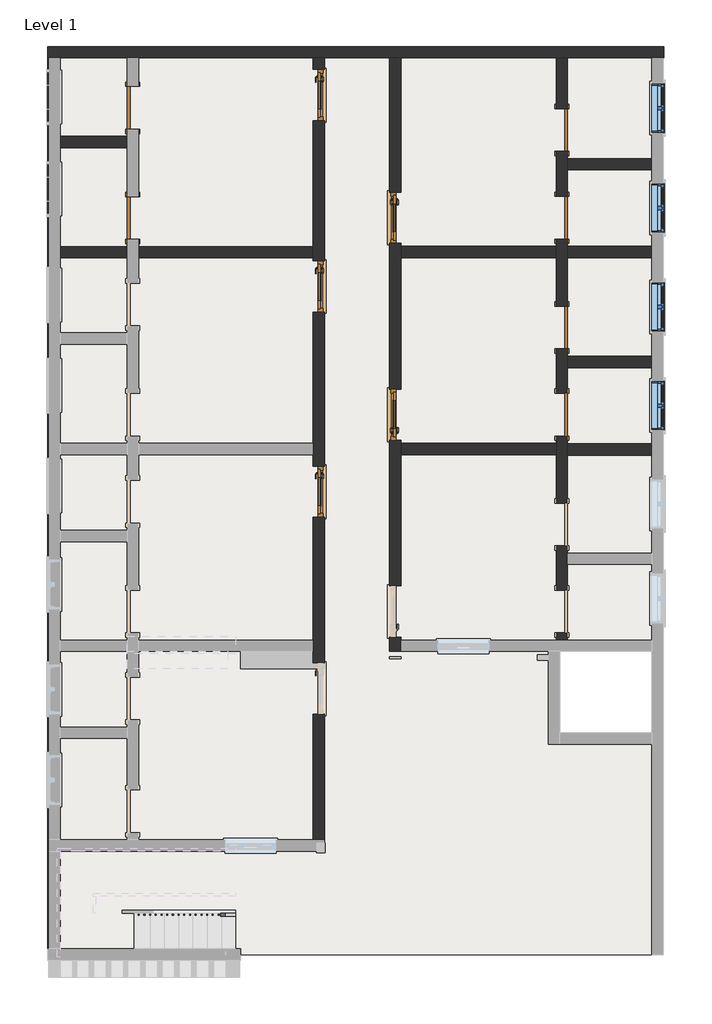
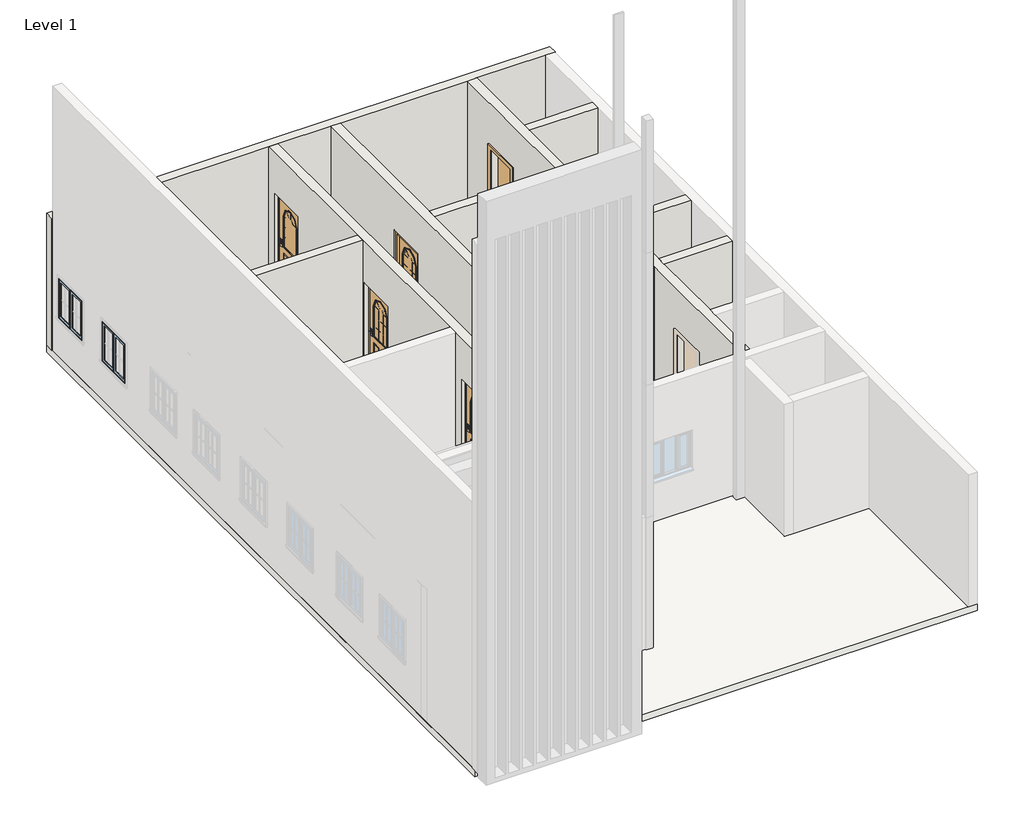
# One storey, part 2 of 4: 13 walls, 11 doors, 6 windows, 1 railing, 1 slab.
"""IFC4 building model written with IfcOpenShell, lengths in millimetres."""

from ifc_helpers import new_model, si_unit, frame, origin, origin_with_axes, place, context, project, spatial, polyline, outline, extrude, faceted_brep, transform, mapped, element, save
from components import doors_extsgl_w_glazing_bars_arched_910x2110mm_1ab485ba, doors_extsgl_w_glazing_bars_arched_910x2110mm_97dcda8a, door_53b1b562, window_c29befe5

model = new_model("IFC4")

# Units and contexts
model_context = context("Model", 3, world=origin())
ifc_project = project(units=[si_unit("LENGTHUNIT", "METRE", prefix="MILLI")], contexts=[model_context])

# Site, building, storey
site = spatial("IfcSite", under=ifc_project)
building = spatial("IfcBuilding", under=site)
storey = spatial("IfcBuildingStorey", under=building, Name="Level 1", Elevation=0.0)

# Doors
placement = place(None, origin())
doors_extsgl_w_glazing_bars_arched_910x2110mm_shape = doors_extsgl_w_glazing_bars_arched_910x2110mm_1ab485ba(model_context)
element("IfcDoor", 1, ObjectType="Doors_ExtSgl_w-Glazing_Bars_Arched : 910x2110mm", at=placement, inside=storey, context=model_context, shape_type="MappedRepresentation", body=[
    mapped(doors_extsgl_w_glazing_bars_arched_910x2110mm_shape, transform((-1635.1108866, 7135.2399728, 0.0), x_axis=(0.0, -1.0, 0.0), y_axis=(1.0, 0.0, 0.0), z_axis=(0.0, 0.0, 1.0))),
])
element("IfcDoor", 2, ObjectType="Doors_ExtSgl_w-Glazing_Bars_Arched : 910x2110mm", at=placement, inside=storey, context=model_context, shape_type="MappedRepresentation", body=[
    mapped(doors_extsgl_w_glazing_bars_arched_910x2110mm_shape, transform((-1635.1108866, 3727.1935874, 0.0), x_axis=(0.0, -1.0, 0.0), y_axis=(1.0, 0.0, 0.0), z_axis=(0.0, 0.0, 1.0))),
])
element("IfcDoor", 3, ObjectType="Doors_ExtSgl_w-Glazing_Bars_Arched : 910x2110mm", at=placement, inside=storey, context=model_context, shape_type="MappedRepresentation", body=[
    mapped(doors_extsgl_w_glazing_bars_arched_910x2110mm_shape, transform((-1635.1108866, 74.0399728, 0.0), x_axis=(0.0, -1.0, 0.0), y_axis=(1.0, 0.0, 0.0), z_axis=(0.0, 0.0, 1.0))),
])
element("IfcDoor", 4, ObjectType="Doors_ExtSgl_w-Glazing_Bars_Arched : 910x2110mm", at=placement, inside=storey, context=model_context, shape_type="MappedRepresentation", body=[
    mapped(doors_extsgl_w_glazing_bars_arched_910x2110mm_shape, transform((-276.2108866, 1445.6399728, 0.0), x_axis=(0.0, 1.0, 0.0), y_axis=(-1.0, 0.0, 0.0), z_axis=(0.0, 0.0, 1.0))),
])
doors_extsgl_w_glazing_bars_arched_910x2110mm_2_shape = doors_extsgl_w_glazing_bars_arched_910x2110mm_97dcda8a(model_context)
element("IfcDoor", 5, ObjectType="Doors_ExtSgl_w-Glazing_Bars_Arched : 910x2110mm", at=placement, inside=storey, context=model_context, shape_type="MappedRepresentation", body=[
    mapped(doors_extsgl_w_glazing_bars_arched_910x2110mm_2_shape, transform((-276.2108866, 4950.8399728, 0.0), x_axis=(0.0, -1.0, 0.0), y_axis=(1.0, 0.0, 0.0), z_axis=(0.0, 0.0, 1.0))),
])
door_shape = door_53b1b562(model_context)
element("IfcDoor", 6, ObjectType="Single-Flush : 30\" x 80\"", at=placement, inside=storey, context=model_context, shape_type="MappedRepresentation", body=[
    mapped(door_shape, transform((-4949.8108866, 6906.6399728, 0.0), x_axis=(0.0, -1.0, 0.0), y_axis=(1.0, 0.0, 0.0), z_axis=(0.0, 0.0, 1.0))),
])
element("IfcDoor", 7, ObjectType="Single-Flush : 30\" x 80\"", at=placement, inside=storey, context=model_context, shape_type="MappedRepresentation", body=[
    mapped(door_shape, transform((-4949.8108866, 4946.3935874, 0.0), x_axis=(0.0, -1.0, 0.0), y_axis=(1.0, 0.0, 0.0), z_axis=(0.0, 0.0, 1.0))),
])
element("IfcDoor", 8, ObjectType="Single-Flush : 30\" x 80\"", at=placement, inside=storey, context=model_context, shape_type="MappedRepresentation", body=[
    mapped(door_shape, transform((2695.5891134, 6512.9399728, 0.0), x_axis=(0.0, 1.0, 0.0), y_axis=(-1.0, 0.0, 0.0), z_axis=(0.0, 0.0, 1.0))),
])
element("IfcDoor", 9, ObjectType="Single-Flush : 30\" x 80\"", at=placement, inside=storey, context=model_context, shape_type="MappedRepresentation", body=[
    mapped(door_shape, transform((2695.5891134, 4950.8399728, 0.0), x_axis=(0.0, 1.0, 0.0), y_axis=(-1.0, 0.0, 0.0), z_axis=(0.0, 0.0, 1.0))),
])
element("IfcDoor", 10, ObjectType="Single-Flush : 30\" x 80\"", at=placement, inside=storey, context=model_context, shape_type="MappedRepresentation", body=[
    mapped(door_shape, transform((2695.5891134, 2995.0399728, 0.0), x_axis=(0.0, 1.0, 0.0), y_axis=(-1.0, 0.0, 0.0), z_axis=(0.0, 0.0, 1.0))),
])
element("IfcDoor", 11, ObjectType="Single-Flush : 30\" x 80\"", at=placement, inside=storey, context=model_context, shape_type="MappedRepresentation", body=[
    mapped(door_shape, transform((2695.5891134, 1445.6399728, 0.0), x_axis=(0.0, 1.0, 0.0), y_axis=(-1.0, 0.0, 0.0), z_axis=(0.0, 0.0, 1.0))),
])

# Railing
element("IfcRailing", 12, ObjectType="Handrail - Rectangular", at=placement, inside=storey, context=model_context, shape_type="SolidModel", body=[
    faceted_brep([(-3117.2664982, -7482.4600272, 1083.7333333), (-3117.2664982, -7482.4600272, 1022.6793317), (-3117.2664982, -7431.6600272, 1022.6793317), (-3117.2664982, -7431.6600272, 1083.7333333), (-5581.0664982, -7482.4600272, 2726.2666667), (-5631.8664982, -7482.4600272, 2699.0793317), (-5631.8664982, -7431.6600272, 2699.0793317), (-5581.0664982, -7431.6600272, 2726.2666667), (-5581.0664982, -7482.4600272, 2777.0666667), (-5631.8664982, -7482.4600272, 2726.2666667), (-5631.8664982, -7431.6600272, 2726.2666667), (-5581.0664982, -7431.6600272, 2777.0666667), (-5708.0664982, -7482.4600272, 2777.0666667), (-5708.0664982, -7482.4600272, 2726.2666667), (-5657.2664982, -7431.6600272, 2726.2666667), (-5657.2664982, -7431.6600272, 2777.0666667), (-5708.0664982, -7355.4600272, 2777.0666667), (-5708.0664982, -7355.4600272, 2726.2666667), (-5657.2664982, -7355.4600272, 2726.2666667), (-5657.2664982, -7355.4600272, 2777.0666667), (-5708.0664982, -7152.2600272, 2777.0666667), (-5708.0664982, -7101.4600272, 2726.2666667), (-5657.2664982, -7101.4600272, 2726.2666667), (-5657.2664982, -7152.2600272, 2777.0666667), (-5708.0664982, -7152.2600272, 2992.12), (-5708.0664982, -7101.4600272, 2941.32), (-5657.2664982, -7101.4600272, 2941.32), (-5657.2664982, -7152.2600272, 2992.12), (-5708.0664982, -7025.2600272, 2992.12), (-5708.0664982, -7025.2600272, 2941.32), (-5657.2664982, -7076.0600272, 2941.32), (-5657.2664982, -7076.0600272, 2992.12), (-5581.0664982, -7025.2600272, 2992.12), (-5566.9957128, -7025.2600272, 2941.32), (-5566.9957128, -7076.0600272, 2941.32), (-5581.0664982, -7076.0600272, 2992.12), (-3117.2664982, -7025.2600272, 4470.4), (-3117.2664982, -7076.0600272, 4470.4), (-3117.2664982, -7076.0600272, 4411.1575287), (-3117.2664982, -7025.2600272, 4411.1575287)], [[[0, 1, 2, 3]], [[1, 0, 4, 5]], [[2, 1, 5, 6]], [[3, 2, 6, 7]], [[0, 3, 7, 4]], [[5, 4, 8, 9]], [[6, 5, 9, 10]], [[7, 6, 10, 11]], [[4, 7, 11, 8]], [[9, 8, 12, 13]], [[10, 9, 13, 14]], [[11, 10, 14, 15]], [[8, 11, 15, 12]], [[13, 12, 16, 17]], [[14, 13, 17, 18]], [[15, 14, 18, 19]], [[12, 15, 19, 16]], [[17, 16, 20, 21]], [[18, 17, 21, 22]], [[19, 18, 22, 23]], [[16, 19, 23, 20]], [[21, 20, 24, 25]], [[22, 21, 25, 26]], [[23, 22, 26, 27]], [[20, 23, 27, 24]], [[25, 24, 28, 29]], [[26, 25, 29, 30]], [[27, 26, 30, 31]], [[24, 27, 31, 28]], [[29, 28, 32, 33]], [[30, 29, 33, 34]], [[31, 30, 34, 35]], [[28, 31, 35, 32]], [[36, 37, 38, 39]], [[33, 32, 36, 39]], [[34, 33, 39, 38]], [[35, 34, 38, 37]], [[32, 35, 37, 36]]]),
    extrude(outline(polyline([(4401.6325287, -3133.1414982), (4390.2025287, -3152.1914982), (3386.6666667, -3152.1914982), (3386.6666667, -3133.1414982), (4401.6325287, -3133.1414982)])), frame((0.0, -7060.1850272, 0.0), z_axis=(0.0, 1.0, 0.0), x_axis=(0.0, 0.0, 1.0)), (0.0, 0.0, 1.0), 19.05),
    extrude(outline(polyline([(4340.6725287, -3234.7414982), (4329.2425287, -3253.7914982), (3386.6666667, -3253.7914982), (3386.6666667, -3234.7414982), (4340.6725287, -3234.7414982)])), frame((0.0, -7060.1850272, 0.0), z_axis=(0.0, 1.0, 0.0), x_axis=(0.0, 0.0, 1.0)), (0.0, 0.0, 1.0), 19.05),
    extrude(outline(polyline([(4279.7125287, -3336.3414982), (4268.2825287, -3355.3914982), (3386.6666667, -3355.3914982), (3386.6666667, -3336.3414982), (4279.7125287, -3336.3414982)])), frame((0.0, -7060.1850272, 0.0), z_axis=(0.0, 1.0, 0.0), x_axis=(0.0, 0.0, 1.0)), (0.0, 0.0, 1.0), 19.05),
    extrude(outline(polyline([(4218.7525287, -3437.9414982), (4207.3225287, -3456.9914982), (3217.3333333, -3456.9914982), (3217.3333333, -3437.9414982), (4218.7525287, -3437.9414982)])), frame((0.0, -7060.1850272, 0.0), z_axis=(0.0, 1.0, 0.0), x_axis=(0.0, 0.0, 1.0)), (0.0, 0.0, 1.0), 19.05),
    extrude(outline(polyline([(4157.7925287, -3539.5414982), (4146.3625287, -3558.5914982), (3217.3333333, -3558.5914982), (3217.3333333, -3539.5414982), (4157.7925287, -3539.5414982)])), frame((0.0, -7060.1850272, 0.0), z_axis=(0.0, 1.0, 0.0), x_axis=(0.0, 0.0, 1.0)), (0.0, 0.0, 1.0), 19.05),
    extrude(outline(polyline([(4096.8325287, -3641.1414982), (4085.4025287, -3660.1914982), (3048.0, -3660.1914982), (3048.0, -3641.1414982), (4096.8325287, -3641.1414982)])), frame((0.0, -7060.1850272, 0.0), z_axis=(0.0, 1.0, 0.0), x_axis=(0.0, 0.0, 1.0)), (0.0, 0.0, 1.0), 19.05),
    extrude(outline(polyline([(4035.8725287, -3742.7414982), (4024.4425287, -3761.7914982), (3048.0, -3761.7914982), (3048.0, -3742.7414982), (4035.8725287, -3742.7414982)])), frame((0.0, -7060.1850272, 0.0), z_axis=(0.0, 1.0, 0.0), x_axis=(0.0, 0.0, 1.0)), (0.0, 0.0, 1.0), 19.05),
    extrude(outline(polyline([(3974.9125287, -3844.3414982), (3963.4825287, -3863.3914982), (3048.0, -3863.3914982), (3048.0, -3844.3414982), (3974.9125287, -3844.3414982)])), frame((0.0, -7060.1850272, 0.0), z_axis=(0.0, 1.0, 0.0), x_axis=(0.0, 0.0, 1.0)), (0.0, 0.0, 1.0), 19.05),
    extrude(outline(polyline([(3913.9525287, -3945.9414982), (3902.5225287, -3964.9914982), (3048.0, -3964.9914982), (3048.0, -3945.9414982), (3913.9525287, -3945.9414982)])), frame((0.0, -7060.1850272, 0.0), z_axis=(0.0, 1.0, 0.0), x_axis=(0.0, 0.0, 1.0)), (0.0, 0.0, 1.0), 19.05),
    extrude(outline(polyline([(3852.9925287, -4047.5414982), (3841.5625287, -4066.5914982), (3048.0, -4066.5914982), (3048.0, -4047.5414982), (3852.9925287, -4047.5414982)])), frame((0.0, -7060.1850272, 0.0), z_axis=(0.0, 1.0, 0.0), x_axis=(0.0, 0.0, 1.0)), (0.0, 0.0, 1.0), 19.05),
    extrude(outline(polyline([(3792.0325287, -4149.1414982), (3780.6025287, -4168.1914982), (2878.6666667, -4168.1914982), (2878.6666667, -4149.1414982), (3792.0325287, -4149.1414982)])), frame((0.0, -7060.1850272, 0.0), z_axis=(0.0, 1.0, 0.0), x_axis=(0.0, 0.0, 1.0)), (0.0, 0.0, 1.0), 19.05),
    extrude(outline(polyline([(3731.0725287, -4250.7414982), (3719.6425287, -4269.7914982), (2878.6666667, -4269.7914982), (2878.6666667, -4250.7414982), (3731.0725287, -4250.7414982)])), frame((0.0, -7060.1850272, 0.0), z_axis=(0.0, 1.0, 0.0), x_axis=(0.0, 0.0, 1.0)), (0.0, 0.0, 1.0), 19.05),
    extrude(outline(polyline([(3670.1125287, -4352.3414982), (3658.6825287, -4371.3914982), (2878.6666667, -4371.3914982), (2878.6666667, -4352.3414982), (3670.1125287, -4352.3414982)])), frame((0.0, -7060.1850272, 0.0), z_axis=(0.0, 1.0, 0.0), x_axis=(0.0, 0.0, 1.0)), (0.0, 0.0, 1.0), 19.05),
    extrude(outline(polyline([(3609.1525287, -4453.9414982), (3597.7225287, -4472.9914982), (2709.3333333, -4472.9914982), (2709.3333333, -4453.9414982), (3609.1525287, -4453.9414982)])), frame((0.0, -7060.1850272, 0.0), z_axis=(0.0, 1.0, 0.0), x_axis=(0.0, 0.0, 1.0)), (0.0, 0.0, 1.0), 19.05),
    extrude(outline(polyline([(3548.1925287, -4555.5414982), (3536.7625287, -4574.5914982), (2709.3333333, -4574.5914982), (2709.3333333, -4555.5414982), (3548.1925287, -4555.5414982)])), frame((0.0, -7060.1850272, 0.0), z_axis=(0.0, 1.0, 0.0), x_axis=(0.0, 0.0, 1.0)), (0.0, 0.0, 1.0), 19.05),
    extrude(outline(polyline([(3487.2325287, -4657.1414982), (3475.8025287, -4676.1914982), (2540.0, -4676.1914982), (2540.0, -4657.1414982), (3487.2325287, -4657.1414982)])), frame((0.0, -7060.1850272, 0.0), z_axis=(0.0, 1.0, 0.0), x_axis=(0.0, 0.0, 1.0)), (0.0, 0.0, 1.0), 19.05),
    extrude(outline(polyline([(3426.2725287, -4758.7414982), (3414.8425287, -4777.7914982), (2540.0, -4777.7914982), (2540.0, -4758.7414982), (3426.2725287, -4758.7414982)])), frame((0.0, -7060.1850272, 0.0), z_axis=(0.0, 1.0, 0.0), x_axis=(0.0, 0.0, 1.0)), (0.0, 0.0, 1.0), 19.05),
    extrude(outline(polyline([(3365.3125287, -4860.3414982), (3353.8825287, -4879.3914982), (2540.0, -4879.3914982), (2540.0, -4860.3414982), (3365.3125287, -4860.3414982)])), frame((0.0, -7060.1850272, 0.0), z_axis=(0.0, 1.0, 0.0), x_axis=(0.0, 0.0, 1.0)), (0.0, 0.0, 1.0), 19.05),
    extrude(outline(polyline([(3304.3525287, -4961.9414982), (3292.9225287, -4980.9914982), (2370.6666667, -4980.9914982), (2370.6666667, -4961.9414982), (3304.3525287, -4961.9414982)])), frame((0.0, -7060.1850272, 0.0), z_axis=(0.0, 1.0, 0.0), x_axis=(0.0, 0.0, 1.0)), (0.0, 0.0, 1.0), 19.05),
    extrude(outline(polyline([(3243.3925287, -5063.5414982), (3231.9625287, -5082.5914982), (2370.6666667, -5082.5914982), (2370.6666667, -5063.5414982), (3243.3925287, -5063.5414982)])), frame((0.0, -7060.1850272, 0.0), z_axis=(0.0, 1.0, 0.0), x_axis=(0.0, 0.0, 1.0)), (0.0, 0.0, 1.0), 19.05),
    extrude(outline(polyline([(3182.4325287, -5165.1414982), (3171.0025287, -5184.1914982), (2201.3333333, -5184.1914982), (2201.3333333, -5165.1414982), (3182.4325287, -5165.1414982)])), frame((0.0, -7060.1850272, 0.0), z_axis=(0.0, 1.0, 0.0), x_axis=(0.0, 0.0, 1.0)), (0.0, 0.0, 1.0), 19.05),
    extrude(outline(polyline([(3121.4725287, -5266.7414982), (3110.0425287, -5285.7914982), (2201.3333333, -5285.7914982), (2201.3333333, -5266.7414982), (3121.4725287, -5266.7414982)])), frame((0.0, -7060.1850272, 0.0), z_axis=(0.0, 1.0, 0.0), x_axis=(0.0, 0.0, 1.0)), (0.0, 0.0, 1.0), 19.05),
    extrude(outline(polyline([(3060.5125287, -5368.3414982), (3049.0825287, -5387.3914982), (2201.3333333, -5387.3914982), (2201.3333333, -5368.3414982), (3060.5125287, -5368.3414982)])), frame((0.0, -7060.1850272, 0.0), z_axis=(0.0, 1.0, 0.0), x_axis=(0.0, 0.0, 1.0)), (0.0, 0.0, 1.0), 19.05),
    extrude(outline(polyline([(2999.5525287, -5469.9414982), (2988.1225287, -5488.9914982), (2032.0, -5488.9914982), (2032.0, -5469.9414982), (2999.5525287, -5469.9414982)])), frame((0.0, -7060.1850272, 0.0), z_axis=(0.0, 1.0, 0.0), x_axis=(0.0, 0.0, 1.0)), (0.0, 0.0, 1.0), 19.05),
    extrude(outline(polyline([(2938.5925287, -5571.5414982), (2927.1625287, -5590.5914982), (2032.0, -5590.5914982), (2032.0, -5571.5414982), (2938.5925287, -5571.5414982)])), frame((0.0, -7060.1850272, 0.0), z_axis=(0.0, 1.0, 0.0), x_axis=(0.0, 0.0, 1.0)), (0.0, 0.0, 1.0), 19.05),
    extrude(outline(polyline([(-5673.1414982, -7161.7850272), (-5692.1914982, -7161.7850272), (-5692.1914982, -7142.7350272), (-5673.1414982, -7142.7350272), (-5673.1414982, -7161.7850272)])), frame((0.0, 0.0, 1862.6666667), z_axis=(0.0, 0.0, 1.0), x_axis=(1.0, 0.0, 0.0)), (0.0, 0.0, 1.0), 863.6),
    extrude(outline(polyline([(-5673.1414982, -7263.3850272), (-5692.1914982, -7263.3850272), (-5692.1914982, -7244.3350272), (-5673.1414982, -7244.3350272), (-5673.1414982, -7263.3850272)])), frame((0.0, 0.0, 1862.6666667), z_axis=(0.0, 0.0, 1.0), x_axis=(1.0, 0.0, 0.0)), (0.0, 0.0, 1.0), 863.6),
    extrude(outline(polyline([(-5673.1414982, -7364.9850272), (-5692.1914982, -7364.9850272), (-5692.1914982, -7345.9350272), (-5673.1414982, -7345.9350272), (-5673.1414982, -7364.9850272)])), frame((0.0, 0.0, 1862.6666667), z_axis=(0.0, 0.0, 1.0), x_axis=(1.0, 0.0, 0.0)), (0.0, 0.0, 1.0), 863.6),
    extrude(outline(polyline([(-5647.7414982, -7447.5350272), (-5647.7414982, -7466.5850272), (-5666.7914982, -7466.5850272), (-5666.7914982, -7447.5350272), (-5647.7414982, -7447.5350272)])), frame((0.0, 0.0, 1862.6666667), z_axis=(0.0, 0.0, 1.0), x_axis=(1.0, 0.0, 0.0)), (0.0, 0.0, 1.0), 863.6),
    extrude(outline(polyline([(2641.9293317, -5546.1414982), (2654.6293317, -5565.1914982), (1693.3333333, -5565.1914982), (1693.3333333, -5546.1414982), (2641.9293317, -5546.1414982)])), frame((0.0, -7466.5850272, 0.0), z_axis=(0.0, 1.0, 0.0), x_axis=(0.0, 0.0, 1.0)), (0.0, 0.0, 1.0), 19.05),
    extrude(outline(polyline([(2574.1959984, -5444.5414982), (2586.8959984, -5463.5914982), (1693.3333333, -5463.5914982), (1693.3333333, -5444.5414982), (2574.1959984, -5444.5414982)])), frame((0.0, -7466.5850272, 0.0), z_axis=(0.0, 1.0, 0.0), x_axis=(0.0, 0.0, 1.0)), (0.0, 0.0, 1.0), 19.05),
    extrude(outline(polyline([(2506.4626651, -5342.9414982), (2519.1626651, -5361.9914982), (1524.0, -5361.9914982), (1524.0, -5342.9414982), (2506.4626651, -5342.9414982)])), frame((0.0, -7466.5850272, 0.0), z_axis=(0.0, 1.0, 0.0), x_axis=(0.0, 0.0, 1.0)), (0.0, 0.0, 1.0), 19.05),
    extrude(outline(polyline([(2438.7293317, -5241.3414982), (2451.4293317, -5260.3914982), (1524.0, -5260.3914982), (1524.0, -5241.3414982), (2438.7293317, -5241.3414982)])), frame((0.0, -7466.5850272, 0.0), z_axis=(0.0, 1.0, 0.0), x_axis=(0.0, 0.0, 1.0)), (0.0, 0.0, 1.0), 19.05),
    extrude(outline(polyline([(2370.9959984, -5139.7414982), (2383.6959984, -5158.7914982), (1524.0, -5158.7914982), (1524.0, -5139.7414982), (2370.9959984, -5139.7414982)])), frame((0.0, -7466.5850272, 0.0), z_axis=(0.0, 1.0, 0.0), x_axis=(0.0, 0.0, 1.0)), (0.0, 0.0, 1.0), 19.05),
    extrude(outline(polyline([(2303.2626651, -5038.1414982), (2315.9626651, -5057.1914982), (1354.6666667, -5057.1914982), (1354.6666667, -5038.1414982), (2303.2626651, -5038.1414982)])), frame((0.0, -7466.5850272, 0.0), z_axis=(0.0, 1.0, 0.0), x_axis=(0.0, 0.0, 1.0)), (0.0, 0.0, 1.0), 19.05),
    extrude(outline(polyline([(2235.5293317, -4936.5414982), (2248.2293317, -4955.5914982), (1354.6666667, -4955.5914982), (1354.6666667, -4936.5414982), (2235.5293317, -4936.5414982)])), frame((0.0, -7466.5850272, 0.0), z_axis=(0.0, 1.0, 0.0), x_axis=(0.0, 0.0, 1.0)), (0.0, 0.0, 1.0), 19.05),
    extrude(outline(polyline([(2167.7959984, -4834.9414982), (2180.4959984, -4853.9914982), (1185.3333333, -4853.9914982), (1185.3333333, -4834.9414982), (2167.7959984, -4834.9414982)])), frame((0.0, -7466.5850272, 0.0), z_axis=(0.0, 1.0, 0.0), x_axis=(0.0, 0.0, 1.0)), (0.0, 0.0, 1.0), 19.05),
    extrude(outline(polyline([(2100.0626651, -4733.3414982), (2112.7626651, -4752.3914982), (1185.3333333, -4752.3914982), (1185.3333333, -4733.3414982), (2100.0626651, -4733.3414982)])), frame((0.0, -7466.5850272, 0.0), z_axis=(0.0, 1.0, 0.0), x_axis=(0.0, 0.0, 1.0)), (0.0, 0.0, 1.0), 19.05),
    extrude(outline(polyline([(2032.3293317, -4631.7414982), (2045.0293317, -4650.7914982), (1185.3333333, -4650.7914982), (1185.3333333, -4631.7414982), (2032.3293317, -4631.7414982)])), frame((0.0, -7466.5850272, 0.0), z_axis=(0.0, 1.0, 0.0), x_axis=(0.0, 0.0, 1.0)), (0.0, 0.0, 1.0), 19.05),
    extrude(outline(polyline([(1964.5959984, -4530.1414982), (1977.2959984, -4549.1914982), (1016.0, -4549.1914982), (1016.0, -4530.1414982), (1964.5959984, -4530.1414982)])), frame((0.0, -7466.5850272, 0.0), z_axis=(0.0, 1.0, 0.0), x_axis=(0.0, 0.0, 1.0)), (0.0, 0.0, 1.0), 19.05),
    extrude(outline(polyline([(1896.8626651, -4428.5414982), (1909.5626651, -4447.5914982), (1016.0, -4447.5914982), (1016.0, -4428.5414982), (1896.8626651, -4428.5414982)])), frame((0.0, -7466.5850272, 0.0), z_axis=(0.0, 1.0, 0.0), x_axis=(0.0, 0.0, 1.0)), (0.0, 0.0, 1.0), 19.05),
    extrude(outline(polyline([(1829.1293317, -4326.9414982), (1841.8293317, -4345.9914982), (846.6666667, -4345.9914982), (846.6666667, -4326.9414982), (1829.1293317, -4326.9414982)])), frame((0.0, -7466.5850272, 0.0), z_axis=(0.0, 1.0, 0.0), x_axis=(0.0, 0.0, 1.0)), (0.0, 0.0, 1.0), 19.05),
    extrude(outline(polyline([(1761.3959984, -4225.3414982), (1774.0959984, -4244.3914982), (846.6666667, -4244.3914982), (846.6666667, -4225.3414982), (1761.3959984, -4225.3414982)])), frame((0.0, -7466.5850272, 0.0), z_axis=(0.0, 1.0, 0.0), x_axis=(0.0, 0.0, 1.0)), (0.0, 0.0, 1.0), 19.05),
    extrude(outline(polyline([(1693.6626651, -4123.7414982), (1706.3626651, -4142.7914982), (846.6666667, -4142.7914982), (846.6666667, -4123.7414982), (1693.6626651, -4123.7414982)])), frame((0.0, -7466.5850272, 0.0), z_axis=(0.0, 1.0, 0.0), x_axis=(0.0, 0.0, 1.0)), (0.0, 0.0, 1.0), 19.05),
    extrude(outline(polyline([(1625.9293317, -4022.1414982), (1638.6293317, -4041.1914982), (677.3333333, -4041.1914982), (677.3333333, -4022.1414982), (1625.9293317, -4022.1414982)])), frame((0.0, -7466.5850272, 0.0), z_axis=(0.0, 1.0, 0.0), x_axis=(0.0, 0.0, 1.0)), (0.0, 0.0, 1.0), 19.05),
    extrude(outline(polyline([(1558.1959984, -3920.5414982), (1570.8959984, -3939.5914982), (677.3333333, -3939.5914982), (677.3333333, -3920.5414982), (1558.1959984, -3920.5414982)])), frame((0.0, -7466.5850272, 0.0), z_axis=(0.0, 1.0, 0.0), x_axis=(0.0, 0.0, 1.0)), (0.0, 0.0, 1.0), 19.05),
    extrude(outline(polyline([(1490.4626651, -3818.9414982), (1503.1626651, -3837.9914982), (508.0, -3837.9914982), (508.0, -3818.9414982), (1490.4626651, -3818.9414982)])), frame((0.0, -7466.5850272, 0.0), z_axis=(0.0, 1.0, 0.0), x_axis=(0.0, 0.0, 1.0)), (0.0, 0.0, 1.0), 19.05),
    extrude(outline(polyline([(1422.7293317, -3717.3414982), (1435.4293317, -3736.3914982), (508.0, -3736.3914982), (508.0, -3717.3414982), (1422.7293317, -3717.3414982)])), frame((0.0, -7466.5850272, 0.0), z_axis=(0.0, 1.0, 0.0), x_axis=(0.0, 0.0, 1.0)), (0.0, 0.0, 1.0), 19.05),
    extrude(outline(polyline([(1354.9959984, -3615.7414982), (1367.6959984, -3634.7914982), (508.0, -3634.7914982), (508.0, -3615.7414982), (1354.9959984, -3615.7414982)])), frame((0.0, -7466.5850272, 0.0), z_axis=(0.0, 1.0, 0.0), x_axis=(0.0, 0.0, 1.0)), (0.0, 0.0, 1.0), 19.05),
    extrude(outline(polyline([(1287.2626651, -3514.1414982), (1299.9626651, -3533.1914982), (338.6666667, -3533.1914982), (338.6666667, -3514.1414982), (1287.2626651, -3514.1414982)])), frame((0.0, -7466.5850272, 0.0), z_axis=(0.0, 1.0, 0.0), x_axis=(0.0, 0.0, 1.0)), (0.0, 0.0, 1.0), 19.05),
    extrude(outline(polyline([(1219.5293317, -3412.5414982), (1232.2293317, -3431.5914982), (338.6666667, -3431.5914982), (338.6666667, -3412.5414982), (1219.5293317, -3412.5414982)])), frame((0.0, -7466.5850272, 0.0), z_axis=(0.0, 1.0, 0.0), x_axis=(0.0, 0.0, 1.0)), (0.0, 0.0, 1.0), 19.05),
    extrude(outline(polyline([(1151.7959984, -3310.9414982), (1164.4959984, -3329.9914982), (169.3333333, -3329.9914982), (169.3333333, -3310.9414982), (1151.7959984, -3310.9414982)])), frame((0.0, -7466.5850272, 0.0), z_axis=(0.0, 1.0, 0.0), x_axis=(0.0, 0.0, 1.0)), (0.0, 0.0, 1.0), 19.05),
    extrude(outline(polyline([(1084.0626651, -3209.3414982), (1096.7626651, -3228.3914982), (169.3333333, -3228.3914982), (169.3333333, -3209.3414982), (1084.0626651, -3209.3414982)])), frame((0.0, -7466.5850272, 0.0), z_axis=(0.0, 1.0, 0.0), x_axis=(0.0, 0.0, 1.0)), (0.0, 0.0, 1.0), 19.05),
    extrude(outline(polyline([(-5673.1414982, -7060.1850272), (-5692.1914982, -7060.1850272), (-5692.1914982, -7041.1350272), (-5673.1414982, -7041.1350272), (-5673.1414982, -7060.1850272)])), frame((0.0, 0.0, 1862.6666667), z_axis=(0.0, 0.0, 1.0), x_axis=(1.0, 0.0, 0.0)), (0.0, 0.0, 1.0), 1078.6533333),
    extrude(outline(polyline([(-5673.1414982, -7447.5350272), (-5673.1414982, -7466.5850272), (-5692.1914982, -7466.5850272), (-5692.1914982, -7447.5350272), (-5673.1414982, -7447.5350272)])), frame((0.0, 0.0, 1862.6666667), z_axis=(0.0, 0.0, 1.0), x_axis=(1.0, 0.0, 0.0)), (0.0, 0.0, 1.0), 863.6),
    extrude(outline(polyline([(4411.1575287, -3117.2664982), (4399.7275287, -3136.3164982), (3386.6666667, -3136.3164982), (3386.6666667, -3117.2664982), (4411.1575287, -3117.2664982)])), frame((0.0, -7060.1850272, 0.0), z_axis=(0.0, 1.0, 0.0), x_axis=(0.0, 0.0, 1.0)), (0.0, 0.0, 1.0), 19.05),
    extrude(outline(polyline([(1022.6793317, -3117.2664982), (1035.3793317, -3136.3164982), (169.3333333, -3136.3164982), (169.3333333, -3117.2664982), (1022.6793317, -3117.2664982)])), frame((0.0, -7466.5850272, 0.0), z_axis=(0.0, 1.0, 0.0), x_axis=(0.0, 0.0, 1.0)), (0.0, 0.0, 1.0), 19.05),
])

# Slab
element("IfcSlab", 13, ObjectType="Generic - 12\"", at=placement, inside=storey, context=model_context, shape_type="SweptSolid", body=[
    extrude(outline(polyline([(4498.9891134, 7998.8399728), (4498.9891134, -8168.2600272), (-6461.1108866, -8168.2600272), (-6461.1108866, 7998.8399728), (4498.9891134, 7998.8399728)]), holes=[polyline([(4295.7891134, -2770.7600272), (2657.4891134, -2770.7600272), (2657.4891134, -4218.5600272), (4295.7891134, -4218.5600272), (4295.7891134, -2770.7600272)])]), frame((0.0, 0.0, -152.4), z_axis=(0.0, 0.0, 1.0), x_axis=(1.0, 0.0, 0.0)), (0.0, 0.0, 1.0), 152.4),
])

# Walls
element("IfcWall", 14, ObjectType="4.5\" p", at=placement, inside=storey, context=model_context, shape_type="SweptSolid", body=[
    extrude(outline(polyline([(-5051.4108866, 6195.4399728), (-6245.2108866, 6195.4399728), (-6245.2108866, 6398.6399728), (-5051.4108866, 6398.6399728), (-5051.4108866, 6195.4399728)])), origin_with_axes(), (0.0, 0.0, 1.0), 3048.0),
])
element("IfcWall", 15, ObjectType="4.5\" p", at=placement, inside=storey, context=model_context, shape_type="SweptSolid", body=[
    extrude(outline(polyline([(-5051.4108866, 4235.1935874), (-6245.2108866, 4235.1935874), (-6245.2108866, 4438.3935874), (-5051.4108866, 4438.3935874), (-5051.4108866, 4235.1935874)])), origin_with_axes(), (0.0, 0.0, 1.0), 3048.0),
])
element("IfcWall", 16, ObjectType="4.5\" p", at=placement, inside=storey, context=model_context, shape_type="Brep", body=[
    faceted_brep([(-1736.7108866, -3886.1600272, 2110.0), (-1736.7108866, -3886.1600272, 0.0), (-1736.7108866, -6123.5600272, 0.0), (-1736.7108866, -6123.5600272, 3048.0), (-1736.7108866, -2770.7600272, 3048.0), (-1736.7108866, -2567.5600272, 3048.0), (-1736.7108866, 734.4399728, 3048.0), (-1736.7108866, 937.6399728, 3048.0), (-1736.7108866, 4235.1935874, 3048.0), (-1736.7108866, 4438.3935874, 3048.0), (-1736.7108866, 7795.6399728, 3048.0), (-1736.7108866, 7795.6399728, 0.0), (-1736.7108866, 7590.2399728, 0.0), (-1736.7108866, 7590.2399728, 2110.0), (-1736.7108866, 6680.2399728, 2110.0), (-1736.7108866, 6680.2399728, 0.0), (-1736.7108866, 4438.3935874, 0.0), (-1736.7108866, 4235.1935874, 0.0), (-1736.7108866, 4182.1935874, 0.0), (-1736.7108866, 4182.1935874, 2110.0), (-1736.7108866, 3272.1935874, 2110.0), (-1736.7108866, 3272.1935874, 0.0), (-1736.7108866, 937.6399728, 0.0), (-1736.7108866, 734.4399728, 0.0), (-1736.7108866, 529.0399728, 0.0), (-1736.7108866, 529.0399728, 2110.0), (-1736.7108866, -380.9600272, 2110.0), (-1736.7108866, -380.9600272, 0.0), (-1736.7108866, -2567.5600272, 0.0), (-1736.7108866, -2770.7600272, 0.0), (-1736.7108866, -2976.1600272, 0.0), (-1736.7108866, -2976.1600272, 2110.0), (-1533.5108866, -6123.5600272, 0.0), (-1533.5108866, -3886.1600272, 0.0), (-1533.5108866, -3886.1600272, 2110.0), (-1533.5108866, -2976.1600272, 2110.0), (-1533.5108866, -2976.1600272, 0.0), (-1533.5108866, -380.9600272, 0.0), (-1533.5108866, -380.9600272, 2110.0), (-1533.5108866, 529.0399728, 2110.0), (-1533.5108866, 529.0399728, 0.0), (-1533.5108866, 3272.1935874, 0.0), (-1533.5108866, 3272.1935874, 2110.0), (-1533.5108866, 4182.1935874, 2110.0), (-1533.5108866, 4182.1935874, 0.0), (-1533.5108866, 6680.2399728, 0.0), (-1533.5108866, 6680.2399728, 2110.0), (-1533.5108866, 7590.2399728, 2110.0), (-1533.5108866, 7590.2399728, 0.0), (-1533.5108866, 7795.6399728, 0.0), (-1533.5108866, 7795.6399728, 3048.0), (-1533.5108866, -6123.5600272, 3048.0)], [[[0, 1, 2, 3, 4, 5, 6, 7, 8, 9, 10, 11, 12, 13, 14, 15, 16, 17, 18, 19, 20, 21, 22, 23, 24, 25, 26, 27, 28, 29, 30, 31]], [[32, 33, 34, 35, 36, 37, 38, 39, 40, 41, 42, 43, 44, 45, 46, 47, 48, 49, 50, 51]], [[12, 11, 49, 48]], [[18, 17, 16, 15, 45, 44]], [[24, 23, 22, 21, 41, 40]], [[2, 1, 33, 32]], [[30, 29, 28, 27, 37, 36]], [[10, 9, 8, 7, 6, 5, 4, 3, 51, 50]], [[3, 2, 32, 51]], [[11, 10, 50, 49]], [[48, 47, 13, 12]], [[46, 45, 15, 14]], [[47, 46, 14, 13]], [[44, 43, 19, 18]], [[42, 41, 21, 20]], [[43, 42, 20, 19]], [[40, 39, 25, 24]], [[38, 37, 27, 26]], [[39, 38, 26, 25]], [[36, 35, 31, 30]], [[34, 33, 1, 0]], [[35, 34, 0, 31]]]),
])
element("IfcWall", 17, ObjectType="4.5\" p", at=placement, inside=storey, context=model_context, shape_type="SweptSolid", body=[
    extrude(outline(polyline([(-1736.7108866, 4235.1935874), (-4848.2108866, 4235.1935874), (-4848.2108866, 4438.3935874), (-1736.7108866, 4438.3935874), (-1736.7108866, 4235.1935874)])), origin_with_axes(), (0.0, 0.0, 1.0), 3048.0),
])
element("IfcWall", 18, ObjectType="4.5\" p", at=placement, inside=storey, context=model_context, shape_type="Brep", body=[
    faceted_brep([(-377.8108866, 4495.8399728, 2110.0), (-377.8108866, 4495.8399728, 0.0), (-377.8108866, 1900.6399728, 0.0), (-377.8108866, 1900.6399728, 2110.0), (-377.8108866, 990.6399728, 2110.0), (-377.8108866, 990.6399728, 0.0), (-377.8108866, -1604.5600272, 0.0), (-377.8108866, -1604.5600272, 2110.0), (-377.8108866, -2514.5600272, 2110.0), (-377.8108866, -2514.5600272, 0.0), (-377.8108866, -2770.7600272, 0.0), (-377.8108866, -2770.7600272, 3048.0), (-377.8108866, 7795.6399728, 3048.0), (-377.8108866, 7795.6399728, 0.0), (-377.8108866, 5405.8399728, 0.0), (-377.8108866, 5405.8399728, 2110.0), (-174.6108866, 1900.6399728, 0.0), (-174.6108866, 4239.6399728, 0.0), (-174.6108866, 4442.8399728, 0.0), (-174.6108866, 4495.8399728, 0.0), (-174.6108866, 4495.8399728, 2110.0), (-174.6108866, 5405.8399728, 2110.0), (-174.6108866, 5405.8399728, 0.0), (-174.6108866, 7795.6399728, 0.0), (-174.6108866, 7795.6399728, 3048.0), (-174.6108866, 4442.8399728, 3048.0), (-174.6108866, 4239.6399728, 3048.0), (-174.6108866, 937.6399728, 3048.0), (-174.6108866, 734.4399728, 3048.0), (-174.6108866, -2770.7600272, 3048.0), (-174.6108866, -2770.7600272, 0.0), (-174.6108866, -2567.5600272, 0.0), (-174.6108866, -2514.5600272, 0.0), (-174.6108866, -2514.5600272, 2110.0), (-174.6108866, -1604.5600272, 2110.0), (-174.6108866, -1604.5600272, 0.0), (-174.6108866, 734.4399728, 0.0), (-174.6108866, 937.6399728, 0.0), (-174.6108866, 990.6399728, 0.0), (-174.6108866, 990.6399728, 2110.0), (-174.6108866, 1900.6399728, 2110.0)], [[[0, 1, 2, 3, 4, 5, 6, 7, 8, 9, 10, 11, 12, 13, 14, 15]], [[16, 17, 18, 19, 20, 21, 22, 23, 24, 25, 26, 27, 28, 29, 30, 31, 32, 33, 34, 35, 36, 37, 38, 39, 40]], [[32, 31, 30, 10, 9]], [[38, 37, 36, 35, 6, 5]], [[14, 13, 23, 22]], [[2, 1, 19, 18, 17, 16]], [[12, 11, 29, 28, 27, 26, 25, 24]], [[13, 12, 24, 23]], [[11, 10, 30, 29]], [[9, 8, 33, 32]], [[7, 6, 35, 34]], [[8, 7, 34, 33]], [[5, 4, 39, 38]], [[3, 2, 16, 40]], [[4, 3, 40, 39]], [[22, 21, 15, 14]], [[20, 19, 1, 0]], [[21, 20, 0, 15]]]),
])
element("IfcWall", 19, ObjectType="4.5\" p", at=placement, inside=storey, context=model_context, shape_type="Brep", body=[
    faceted_brep([(2593.9891134, -2440.5600272, 2032.0), (2593.9891134, -2440.5600272, 0.0), (2593.9891134, -2567.5600272, 0.0), (2593.9891134, -2567.5600272, 3048.0), (2593.9891134, 734.4399728, 3048.0), (2593.9891134, 937.6399728, 3048.0), (2593.9891134, 4239.6399728, 3048.0), (2593.9891134, 4442.8399728, 3048.0), (2593.9891134, 7795.6399728, 3048.0), (2593.9891134, 7795.6399728, 0.0), (2593.9891134, 6893.9399728, 0.0), (2593.9891134, 6893.9399728, 2032.0), (2593.9891134, 6131.9399728, 2032.0), (2593.9891134, 6131.9399728, 0.0), (2593.9891134, 5331.8399728, 0.0), (2593.9891134, 5331.8399728, 2032.0), (2593.9891134, 4569.8399728, 2032.0), (2593.9891134, 4569.8399728, 0.0), (2593.9891134, 4442.8399728, 0.0), (2593.9891134, 4239.6399728, 0.0), (2593.9891134, 3376.0399728, 0.0), (2593.9891134, 3376.0399728, 2032.0), (2593.9891134, 2614.0399728, 2032.0), (2593.9891134, 2614.0399728, 0.0), (2593.9891134, 1826.6399728, 0.0), (2593.9891134, 1826.6399728, 2032.0), (2593.9891134, 1064.6399728, 2032.0), (2593.9891134, 1064.6399728, 0.0), (2593.9891134, 937.6399728, 0.0), (2593.9891134, 734.4399728, 0.0), (2593.9891134, -129.1600272, 0.0), (2593.9891134, -129.1600272, 2032.0), (2593.9891134, -891.1600272, 2032.0), (2593.9891134, -891.1600272, 0.0), (2593.9891134, -1678.5600272, 0.0), (2593.9891134, -1678.5600272, 2032.0), (2797.1891134, -2567.5600272, 0.0), (2797.1891134, -2440.5600272, 0.0), (2797.1891134, -2440.5600272, 2032.0), (2797.1891134, -1678.5600272, 2032.0), (2797.1891134, -1678.5600272, 0.0), (2797.1891134, -1221.3600272, 0.0), (2797.1891134, -1018.1600272, 0.0), (2797.1891134, -891.1600272, 0.0), (2797.1891134, -891.1600272, 2032.0), (2797.1891134, -129.1600272, 2032.0), (2797.1891134, -129.1600272, 0.0), (2797.1891134, 721.7399728, 0.0), (2797.1891134, 924.9399728, 0.0), (2797.1891134, 1064.6399728, 0.0), (2797.1891134, 1064.6399728, 2032.0), (2797.1891134, 1826.6399728, 2032.0), (2797.1891134, 1826.6399728, 0.0), (2797.1891134, 2283.8399728, 0.0), (2797.1891134, 2487.0399728, 0.0), (2797.1891134, 2614.0399728, 0.0), (2797.1891134, 2614.0399728, 2032.0), (2797.1891134, 3376.0399728, 2032.0), (2797.1891134, 3376.0399728, 0.0), (2797.1891134, 4239.6399728, 0.0), (2797.1891134, 4442.8399728, 0.0), (2797.1891134, 4569.8399728, 0.0), (2797.1891134, 4569.8399728, 2032.0), (2797.1891134, 5331.8399728, 2032.0), (2797.1891134, 5331.8399728, 0.0), (2797.1891134, 5801.7399728, 0.0), (2797.1891134, 6004.9399728, 0.0), (2797.1891134, 6131.9399728, 0.0), (2797.1891134, 6131.9399728, 2032.0), (2797.1891134, 6893.9399728, 2032.0), (2797.1891134, 6893.9399728, 0.0), (2797.1891134, 7795.6399728, 0.0), (2797.1891134, 7795.6399728, 3048.0), (2797.1891134, 6004.9399728, 3048.0), (2797.1891134, 5801.7399728, 3048.0), (2797.1891134, 4442.8399728, 3048.0), (2797.1891134, 4239.6399728, 3048.0), (2797.1891134, 2487.0399728, 3048.0), (2797.1891134, 2283.8399728, 3048.0), (2797.1891134, 924.9399728, 3048.0), (2797.1891134, 721.7399728, 3048.0), (2797.1891134, -1018.1600272, 3048.0), (2797.1891134, -1221.3600272, 3048.0), (2797.1891134, -2567.5600272, 3048.0)], [[[0, 1, 2, 3, 4, 5, 6, 7, 8, 9, 10, 11, 12, 13, 14, 15, 16, 17, 18, 19, 20, 21, 22, 23, 24, 25, 26, 27, 28, 29, 30, 31, 32, 33, 34, 35]], [[36, 37, 38, 39, 40, 41, 42, 43, 44, 45, 46, 47, 48, 49, 50, 51, 52, 53, 54, 55, 56, 57, 58, 59, 60, 61, 62, 63, 64, 65, 66, 67, 68, 69, 70, 71, 72, 73, 74, 75, 76, 77, 78, 79, 80, 81, 82, 83]], [[71, 70, 10, 9]], [[67, 66, 65, 64, 14, 13]], [[61, 60, 59, 58, 20, 19, 18, 17]], [[55, 54, 53, 52, 24, 23]], [[30, 29, 28, 27, 49, 48, 47, 46]], [[34, 33, 43, 42, 41, 40]], [[2, 1, 37, 36]], [[8, 7, 6, 5, 4, 3, 83, 82, 81, 80, 79, 78, 77, 76, 75, 74, 73, 72]], [[9, 8, 72, 71]], [[3, 2, 36, 83]], [[11, 10, 70, 69]], [[12, 11, 69, 68]], [[13, 12, 68, 67]], [[15, 14, 64, 63]], [[16, 15, 63, 62]], [[17, 16, 62, 61]], [[21, 20, 58, 57]], [[22, 21, 57, 56]], [[23, 22, 56, 55]], [[25, 24, 52, 51]], [[26, 25, 51, 50]], [[27, 26, 50, 49]], [[44, 43, 33, 32]], [[45, 44, 32, 31]], [[46, 45, 31, 30]], [[38, 37, 1, 0]], [[39, 38, 0, 35]], [[40, 39, 35, 34]]]),
])
element("IfcWall", 20, ObjectType="4.5\" p", at=placement, inside=storey, context=model_context, shape_type="SweptSolid", body=[
    extrude(outline(polyline([(4295.7891134, 5801.7399728), (2797.1891134, 5801.7399728), (2797.1891134, 6004.9399728), (4295.7891134, 6004.9399728), (4295.7891134, 5801.7399728)])), origin_with_axes(), (0.0, 0.0, 1.0), 3048.0),
])
element("IfcWall", 21, ObjectType="4.5\" p", at=placement, inside=storey, context=model_context, shape_type="SweptSolid", body=[
    extrude(outline(polyline([(4295.7891134, 4239.6399728), (2797.1891134, 4239.6399728), (2797.1891134, 4442.8399728), (4295.7891134, 4442.8399728), (4295.7891134, 4239.6399728)])), origin_with_axes(), (0.0, 0.0, 1.0), 3048.0),
])
element("IfcWall", 22, ObjectType="4.5\" p", at=placement, inside=storey, context=model_context, shape_type="SweptSolid", body=[
    extrude(outline(polyline([(4295.7891134, 2283.8399728), (2797.1891134, 2283.8399728), (2797.1891134, 2487.0399728), (4295.7891134, 2487.0399728), (4295.7891134, 2283.8399728)])), origin_with_axes(), (0.0, 0.0, 1.0), 3048.0),
])
element("IfcWall", 23, ObjectType="4.5\" p", at=placement, inside=storey, context=model_context, shape_type="SweptSolid", body=[
    extrude(outline(polyline([(4295.7891134, 721.7399728), (2797.1891134, 721.7399728), (2797.1891134, 924.9399728), (4295.7891134, 924.9399728), (4295.7891134, 721.7399728)])), origin_with_axes(), (0.0, 0.0, 1.0), 3048.0),
])
element("IfcWall", 24, ObjectType="4.5\" p", at=placement, inside=storey, context=model_context, shape_type="SweptSolid", body=[
    extrude(outline(polyline([(2593.9891134, 4239.6399728), (-174.6108866, 4239.6399728), (-174.6108866, 4442.8399728), (2593.9891134, 4442.8399728), (2593.9891134, 4239.6399728)])), origin_with_axes(), (0.0, 0.0, 1.0), 3048.0),
])
element("IfcWall", 25, ObjectType="4.5\" p", at=placement, inside=storey, context=model_context, shape_type="SweptSolid", body=[
    extrude(outline(polyline([(2593.9891134, 734.4399728), (-174.6108866, 734.4399728), (-174.6108866, 937.6399728), (2593.9891134, 937.6399728), (2593.9891134, 734.4399728)])), origin_with_axes(), (0.0, 0.0, 1.0), 3048.0),
])
element("IfcWall", 26, ObjectType="9\" w", at=placement, inside=storey, context=model_context, shape_type="Brep", body=[
    faceted_brep([(-6461.1108866, 7795.6399728, 0.0), (-6448.4108866, 7795.6399728, 0.0), (-6245.2108866, 7795.6399728, 0.0), (-5051.4108866, 7795.6399728, 0.0), (-4848.2108866, 7795.6399728, 0.0), (-1736.7108866, 7795.6399728, 0.0), (-1533.5108866, 7795.6399728, 0.0), (-377.8108866, 7795.6399728, 0.0), (-174.6108866, 7795.6399728, 0.0), (2593.9891134, 7795.6399728, 0.0), (2797.1891134, 7795.6399728, 0.0), (4295.7891134, 7795.6399728, 0.0), (4498.9891134, 7795.6399728, 0.0), (4511.6891134, 7795.6399728, 0.0), (4511.6891134, 7795.6399728, 3048.0), (4498.9891134, 7795.6399728, 3048.0), (4295.7891134, 7795.6399728, 3048.0), (2797.1891134, 7795.6399728, 3048.0), (2593.9891134, 7795.6399728, 3048.0), (-174.6108866, 7795.6399728, 3048.0), (-377.8108866, 7795.6399728, 3048.0), (-1533.5108866, 7795.6399728, 3048.0), (-1736.7108866, 7795.6399728, 3048.0), (-4848.2108866, 7795.6399728, 3048.0), (-5051.4108866, 7795.6399728, 3048.0), (-6245.2108866, 7795.6399728, 3048.0), (-6448.4108866, 7795.6399728, 3048.0), (-6461.1108866, 7795.6399728, 3048.0), (-6461.1108866, 7998.8399728, 0.0), (-6461.1108866, 7998.8399728, 3048.0), (4511.6891134, 7998.8399728, 3048.0), (4511.6891134, 7998.8399728, 0.0)], [[[0, 1, 2, 3, 4, 5, 6, 7, 8, 9, 10, 11, 12, 13, 14, 15, 16, 17, 18, 19, 20, 21, 22, 23, 24, 25, 26, 27]], [[28, 29, 30, 31]], [[13, 12, 11, 10, 9, 8, 7, 6, 5, 4, 3, 2, 1, 0, 28, 31]], [[14, 13, 31, 30]], [[27, 26, 25, 24, 23, 22, 21, 20, 19, 18, 17, 16, 15, 14, 30, 29]], [[0, 27, 29, 28]]]),
])

# Windows
window_shape = window_c29befe5(model_context)
element("IfcWindow", 27, ObjectType="Window-Casement-Double : 34\" x 36\"", at=placement, inside=storey, context=model_context, shape_type="MappedRepresentation", body=[
    mapped(window_shape, transform((-6346.8108866, 7097.1399728, 0.0), x_axis=(0.0, 1.0, 0.0), y_axis=(-1.0, 0.0, 0.0), z_axis=(0.0, 0.0, 1.0))),
])
element("IfcWindow", 28, ObjectType="Window-Casement-Double : 34\" x 36\"", at=placement, inside=storey, context=model_context, shape_type="MappedRepresentation", body=[
    mapped(window_shape, transform((-6346.8108866, 5458.8399728, 0.0), x_axis=(0.0, 1.0, 0.0), y_axis=(-1.0, 0.0, 0.0), z_axis=(0.0, 0.0, 1.0))),
])
element("IfcWindow", 29, ObjectType="Window-Casement-Double : 34\" x 36\"", at=placement, inside=storey, context=model_context, shape_type="MappedRepresentation", body=[
    mapped(window_shape, transform((4397.3891134, 1604.3899728, 0.0), x_axis=(0.0, -1.0, 0.0), y_axis=(1.0, 0.0, 0.0), z_axis=(0.0, 0.0, 1.0))),
])
element("IfcWindow", 30, ObjectType="Window-Casement-Double : 34\" x 36\"", at=placement, inside=storey, context=model_context, shape_type="MappedRepresentation", body=[
    mapped(window_shape, transform((4397.3891134, 3363.3399728, 0.0), x_axis=(0.0, -1.0, 0.0), y_axis=(1.0, 0.0, 0.0), z_axis=(0.0, 0.0, 1.0))),
])
element("IfcWindow", 31, ObjectType="Window-Casement-Double : 34\" x 36\"", at=placement, inside=storey, context=model_context, shape_type="MappedRepresentation", body=[
    mapped(window_shape, transform((4397.3891134, 5122.2899728, 0.0), x_axis=(0.0, -1.0, 0.0), y_axis=(1.0, 0.0, 0.0), z_axis=(0.0, 0.0, 1.0))),
])
element("IfcWindow", 32, ObjectType="Window-Casement-Double : 34\" x 36\"", at=placement, inside=storey, context=model_context, shape_type="MappedRepresentation", body=[
    mapped(window_shape, transform((4397.3891134, 6900.2899728, 0.0), x_axis=(0.0, -1.0, 0.0), y_axis=(1.0, 0.0, 0.0), z_axis=(0.0, 0.0, 1.0))),
])

save(model, "model.ifc")

# Revit data of these elements
# Type "Doors_ExtSgl_w-Glazing_Bars_Arched : 910x2110mm"
#   Type Mark = "19"
#   Type Comments = "External Single"
#   Operation = "SingleSwingRight"
#   Construction Type Id = "SGL"
#   Keynote = "L20"
#   Analytic Construction = "Large single-glazed windows"
#   Wrap Layers (Int) from Ext = 0' - 6.98819"
#   Wrap Layers (Ext) from Ext = 0' - 4.03543"
#   Visual Light Transmittance = 0.9
#   Thickness = 0' - 1.73228"
#   Solar Heat Gain Coefficient = 0.86
#   Rough Width = 2' - 11.82677"
#   Rough Height = 6' - 11.07087"
#   O/A Frame Width = 0' - 2.51969"
#   Heat Transfer Coefficient (U) = 0.979472 BTU/(h·ft²·°F)
#   Handle Z Distance = 3' - 5.33858"
#   Glazing Thickness = 0' - 0.94488"
#   FrameWidth = 0' - 1.65354"
#   FrameOffset - External = 0' - 0.98425"
#   FrameDepth = 0' - 3.50394"
#   Door Panel Width = 2' - 7.77165"
#   Door Panel Thickness = 0' - 1.73228"
#   Door Panel Height = 6' - 6.74016"
#   DONT CHANGE - Half Glazed Width = 0' - 9.98031"
#   DONT CHANGE - Glazed Width = 1' - 7.96063"
#   Cill Thickness = 0' - 2.14567"
#   Cill Projection = 0' - 1.1811"
#   Handle X Distance = 0' - 2.95276"
#   Height = 6' - 11.07087"
#   Structural Tolerance = 0' - 0.25591"
#   Tolerance = 0' - 0.11811"
#   Undercut = 0' - 0.15748"
#   Width = 2' - 11.82677"
#   Cill Extension = 0' - 0.98425"
#   Cavity Closer Width = 0' - 1.9685"
#   Cavity Closer Offset from Ext = 0' - 4.03543"
#   Cavity Closer Depth = 0' - 3.34646"
#   Vis - Ironmongery = yes
#   Vis - Glazing Bars = yes
#   Vis - Cavity Closers = yes
#   Define Thermal Properties by = 1
#   Function = 1
#   Material Glass = Door - Glazing
#   Material Glazing Bar = Door - Panel
#   Material Door = Door - Panel
#   Material Frame = Door - Frame/Mullion
#   Material Ironmongery = Door - Handle
#   Wall Closure = (empty or 0)
# Type "Single-Flush : 30\" x 80\""
#   Type Mark = "5"
#   Construction Type Id = "MDOOR"
#   Assembly Code = "C1020"
#   Analytic Construction = "Metal"
#   Thickness = 0' - 2"
#   Heat Transfer Coefficient (U) = 0.651978 BTU/(h·ft²·°F)
#   Height = 6' - 8"
#   Trim Projection Ext = 0' - 1"
#   Trim Projection Int = 0' - 1"
#   Trim Width = 0' - 3"
#   Width = 2' - 6"
#   Define Thermal Properties by = 1
#   Define Thermal Properties by = 1
#   Door Material = Door - Panel
#   Frame Material = Door - Frame
#   Visual Light Transmittance = 0
#   Solar Heat Gain Coefficient = 0
#   Function = (empty or 0)
#   Wall Closure = (empty or 0)
# Type "Handrail - Rectangular"
#   Assembly Code = "C2010400"
#   built-in parameter 1008612 = 0.0416667 (stored number, unit not read)
#   built-in parameter 1008611 = 0.0416667 (stored number, unit not read)
#   built-in parameter 1008609 = 0.333333 (stored number, unit not read)
#   built-in parameter 1008604 = 0.166667 (stored number, unit not read)
#   built-in parameter 1008603 = 0.166667 (stored number, unit not read)
#   Railing Height = 3' - 0"
#   built-in parameter 1008630 = 2
#   built-in parameter 1008610 = 2
#   built-in parameter 1008618 = Baluster - Square : 3/4"
# Type "Generic - 12\""
#   Assembly Code = "B1010"
#   Function = 0
#   Layers, outside or top first: 0' - 6" no material (function 1)
# Type "4.5\" p"
#   Assembly Code = "B2010"
#   Layers, outside or top first: 0' - 8" no material (function 1)
# Type "9\" w"
#   Assembly Code = "B2010"
#   Layers, outside or top first: 0' - 8" no material (function 1)
# Type "Window-Casement-Double : 34\" x 36\""
#   Type Mark = "14"
#   Fire Rating = "0.5h"
#   Assembly Code = "B2020100"
#   Analytic Construction = "Double glazing - domestic"
#   Frame Extension [instance default] = 0' - 0 1/4"
#   Window Inset [instance default] = 0' - 0"
#   Wall Thickness [instance default] = 0' - 6"
#   Interior Wall Closure [instance default] = 0' - 2 1/4"
#   Half Width = 1' - 5"
#   Visual Light Transmittance = 0.81
#   Thermal Resistance (R) = 1.8146 (h·ft²·°F)/BTU
#   Solar Heat Gain Coefficient = 0.76
#   Rough Width = 2' - 10 1/2"
#   Rough Height = 3' - 0 1/2"
#   Height = 3' - 0"
#   Heat Transfer Coefficient (U) = 0.5511 BTU/(h·ft²·°F)
#   Exterior Wall Closure [instance default] = 0' - 1 1/4"
#   Extension Jamb [instance default] = 0' - 2 1/4"
#   Default Sill Height = 3' - 0"
#   Width = 2' - 10"
#   Define Thermal Properties by = 0
#   Muntin Visibility = yes
#   Interior Trim Visibility [instance default] = yes
#   Exterior Trim Visibility [instance default] = yes
#   Extension Jamb Visibility [instance default] = yes
#   Interior Trim Material = Wood - Stained
#   Muntin Pattern = Muntin Pattern_2x2 : Muntin Pattern_2x2
#   Interior Trim = Trim-Window-Interior-Flat : Picture Frame
#   Interior Frame Material = Wood - Stained
#   Glass Panel Material = Glass
#   Exterior Trim Material = Clad - White
#   Exterior Trim = Trim-Window-Exterior-Flat : with Sill
#   Exterior Frame Material = Clad - White
#   Wall Closure = (empty or 0)
# Elements 1, 2, 3, 4, 5 (IfcDoor, "Doors_ExtSgl_w-Glazing_Bars_Arched : 910x2110mm")
#   Phase Created = New Construction
#   Materials on its faces: "Door - Panel", "Door - Handle", "Door - Frame/Mullion", "Door - Glazing"
# Elements 6, 7, 8, 9, 10, 11 (IfcDoor, "Single-Flush : 30\" x 80\"")
#   Phase Created = New Construction
#   Materials on its faces: "Door - Frame", "Door - Panel"
# Element 12 (IfcRailing, "Handrail - Rectangular")
#   Phase Created = New Construction
# Element 13 (IfcSlab, "Generic - 12\"")
#   Height Offset From Level = 0' - 0"
#   Phase Created = New Construction
#   Materials on its faces: "Default Floor", "Grass", "Earth", "Wood - Stained"
# Elements 14, 15, 17, 19, 20, 21, 22, 23, 24, 25 (IfcWall, "4.5\" p")
#   Top Offset = 0' - 0"
#   Base Offset = 0' - 0"
#   wall height = 10' - 0"
#   Phase Created = New Construction
#   Base Constraint = Level 1
#   Top Constraint = Level 2
#   Materials on its faces: "Default Wall"
# Element 16 (IfcWall, "4.5\" p")
#   Top Offset = 0' - 0"
#   Base Offset = 0' - 0"
#   wall height = 10' - 0"
#   Phase Created = New Construction
#   Base Constraint = Level 1
#   Top Constraint = Level 2
#   Materials on its faces: "Default Wall", "Brick, Common"
# Element 18 (IfcWall, "4.5\" p")
#   Top Offset = 0' - 0"
#   Base Offset = 0' - 0"
#   wall height = 10' - 0"
#   Phase Created = New Construction
#   Base Constraint = Level 1
#   Top Constraint = Level 2
#   Materials on its faces: "Default Wall", "Brick, Common", "Window Frame"
# Element 26 (IfcWall, "9\" w")
#   Top Offset = 0' - 0"
#   Base Offset = 0' - 0"
#   wall height = 10' - 0"
#   Phase Created = New Construction
#   Base Constraint = Level 1
#   Top Constraint = Level 2
#   Materials on its faces: "Default Wall", "Cherry", "Wood - Stained"
# Element 27 (IfcWindow, "Window-Casement-Double : 34\" x 36\"")
#   Mark = "1"
#   Window Inset = 0' - 0"
#   Interior Wall Closure = 0' - 2 1/4"
#   Frame Extension = 0' - 0 1/4"
#   Exterior Wall Closure = 0' - 1 1/4"
#   Interior Trim Visibility = yes
#   Exterior Trim Visibility = yes
#   Phase Created = New Construction
#   Materials on its faces: "Wood - Stained", "Glass", "Clad - White"
# Element 28 (IfcWindow, "Window-Casement-Double : 34\" x 36\"")
#   Mark = "2"
#   Window Inset = 0' - 0"
#   Interior Wall Closure = 0' - 2 1/4"
#   Frame Extension = 0' - 0 1/4"
#   Exterior Wall Closure = 0' - 1 1/4"
#   Interior Trim Visibility = yes
#   Exterior Trim Visibility = yes
#   Phase Created = New Construction
#   Materials on its faces: "Wood - Stained", "Glass", "Clad - White"
# Element 29 (IfcWindow, "Window-Casement-Double : 34\" x 36\"")
#   Mark = "11"
#   Window Inset = 0' - 0"
#   Interior Wall Closure = 0' - 2 1/4"
#   Frame Extension = 0' - 0 1/4"
#   Exterior Wall Closure = 0' - 1 1/4"
#   Interior Trim Visibility = yes
#   Exterior Trim Visibility = yes
#   Phase Created = New Construction
#   Materials on its faces: "Wood - Stained", "Glass", "Clad - White"
# Element 30 (IfcWindow, "Window-Casement-Double : 34\" x 36\"")
#   Mark = "12"
#   Window Inset = 0' - 0"
#   Interior Wall Closure = 0' - 2 1/4"
#   Frame Extension = 0' - 0 1/4"
#   Exterior Wall Closure = 0' - 1 1/4"
#   Interior Trim Visibility = yes
#   Exterior Trim Visibility = yes
#   Phase Created = New Construction
#   Materials on its faces: "Wood - Stained", "Glass", "Clad - White"
# Element 31 (IfcWindow, "Window-Casement-Double : 34\" x 36\"")
#   Mark = "13"
#   Window Inset = 0' - 0"
#   Interior Wall Closure = 0' - 2 1/4"
#   Frame Extension = 0' - 0 1/4"
#   Exterior Wall Closure = 0' - 1 1/4"
#   Interior Trim Visibility = yes
#   Exterior Trim Visibility = yes
#   Phase Created = New Construction
#   Materials on its faces: "Wood - Stained", "Glass", "Clad - White"
# Element 32 (IfcWindow, "Window-Casement-Double : 34\" x 36\"")
#   Mark = "14"
#   Window Inset = 0' - 0"
#   Interior Wall Closure = 0' - 2 1/4"
#   Frame Extension = 0' - 0 1/4"
#   Exterior Wall Closure = 0' - 1 1/4"
#   Interior Trim Visibility = yes
#   Exterior Trim Visibility = yes
#   Phase Created = New Construction
#   Materials on its faces: "Wood - Stained", "Glass", "Clad - White"
# Materials
#   "Door - Glazing": colour RGB 0 0 255, transparency 0.75
#   "Door - Panel": class "Wood", colour RGB 210 159 95, transparency 0, Cost = 0
#   "Door - Frame/Mullion": class "Wood", colour RGB 212 179 113, transparency 0
#   "Door - Handle": colour RGB 247 247 247, transparency 0
#   "Door - Frame": colour RGB 118 70 51, transparency 0, Cost = 0
#   "Wood - Stained": class "Wood", colour RGB 224 178 126, transparency 0, Cost = 0
#   "Glass": class "Glass", colour RGB 0 128 192, transparency 0.75, Description = "Soda Lime Glass", Cost = 0
#   "Clad - White": class "Wood", colour RGB 242 242 238, transparency 0, Cost = 0
#   "Default Floor": colour RGB 128 128 128, transparency 0, Cost = 0
#   "Grass": class "Generic", colour RGB 104 137 66, transparency 0, Description = "Physical material.", Cost = 0
#   "Earth": class "Generic", colour RGB 97 75 62, transparency 0, Description = "Soil", Cost = 0
#   "Default Wall": colour RGB 128 128 128, transparency 0, Cost = 0
#   "Brick, Common": class "Masonry", colour RGB 170 98 104, transparency 0, Description = "Common brick", Cost = 0
#   "Window Frame": colour RGB 249 249 249, transparency 0
#   "Cherry": class "Wood", colour RGB 226 177 128, transparency 0, Description = "Prunus Serotina", Cost = 0
